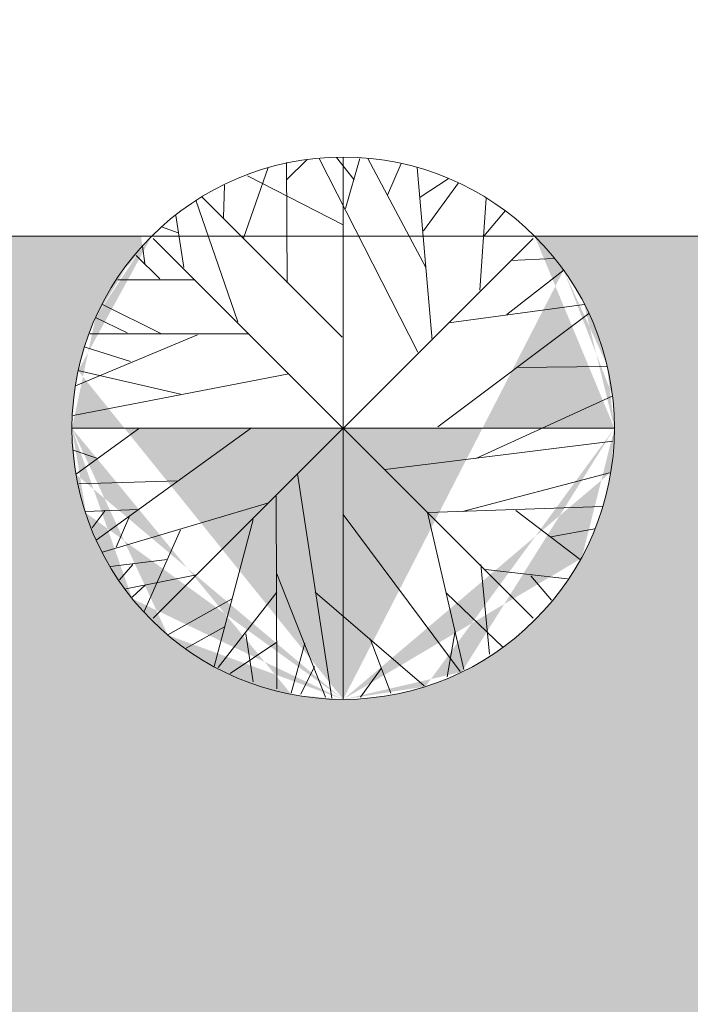
# Model space of a CAD drawing. Units: inches. Extents: x 459864 to 460310, y 324185 to 324787.
# Tile 62 of 112: x 460180 to 460210, y 324239 to 324282. Entities that reach past the tile are written whole.
import ezdxf

# ---------------------------------------------------------------- set-up
doc = ezdxf.new("R2010")
doc.units = ezdxf.units.IN
doc.layers.add('L-PLNT', color=3, linetype='Continuous', lineweight=13)
doc.layers.add('L-SITE-PATT', color=252, linetype='Continuous', lineweight=13)

# ---------------------------------------------------------------- blocks, each defined once
blk = doc.blocks.new('Tree - deciduous plan')
for p, q in [((-12.5388, 54.9406), (-7.9613, 59.4546)), ((-5.3205, 59.6806), (16.5105, 16.7963)), ((2.426, 54.9406), (-1.4472, 59.9056)), ((0, 59.9996), (0, -60)), ((0.4894, 48.6208), (3.6584, 59.6806)), ((18.2711, 35.5298), (5.419, 59.6806)), ((-22.0458, 42.0753), (-16.5881, 57.6486)), ((-12.3627, 32.1443), (-12.5388, 58.7776)), ((9.8203, 51.5549), (12.8133, 58.5516)), ((19.6795, 19.5047), (16.3344, 57.6486)), ((-21.1656, 55.8436), (-0.0388, 45.0094)), ((17.0387, 51.1035), (23.2006, 55.1666)), ((-26.4472, 46.5894), (-26.2712, 53.8116)), ((17.7429, 43.6552), (25.4894, 54.2636)), ((-32.6092, 50.4264), (-23.2782, 23.5674)), ((-31.2008, 51.1035), (-0.2149, 20.1818)), ((31.6513, 50.8778), (30.2429, 30.5643)), ((31.1232, 42.5267), (35.8767, 48.1693)), ((-37.0107, 47.0408), (-35.25, 35.5298)), ((-40.1797, 44.558), (-36.4825, 43.2038)), ((42, 42), (-42, -42)), ((42, -42), (-42, 42)), ((-43.8768, 36.4326), (-44.405, 40.2696)), ((-45.8134, 38.2383), (-40.5318, 33.0471)), ((37.1091, 37.1098), (46.6161, 37.5612)), ((36.2288, 25.1474), (48.9049, 35.0784)), ((-49.8627, 32.8214), (-32.7853, 32.8214)), ((-53.2078, 27.4044), (-40.1797, 20.859)), ((23.3767, 23.3417), (53.3063, 27.4044)), ((-54.7923, 24.4702), (-47.75, 21.0847)), ((54.3626, 25.3731), (20.9119, 0.3198)), ((-32.2571, 20.6333), (-59.1937, 9.348)), ((-56.0247, 20.859), (-20.8134, 20.859)), ((-57.081, 17.9248), (-47.0458, 14.7649)), ((38.5175, 13.4107), (58.2359, 13.6364)), ((-59.7219, 2.8025), (-12.0106, 12.0565)), ((-58.6656, 12.7336), (-35.9543, 7.5424)), ((29.3626, -6.6771), (59.4682, 7.091)), ((-54.6162, -24.7335), (-20.2853, 0.0941)), ((-60, 0), (60, 0)), ((-45.2853, -0.1316), (-59.0177, -10.0627)), ((9.2922, -9.1598), (59.6443, -2.8401)), ((-59.7219, -4.8714), (-54.2641, -6.6771)), ((-10.074, -10.0627), (-2.5036, -59.7178)), ((26.3697, -18.4138), (58.9401, -9.8369)), ((-58.4895, -12.3197), (-36.4825, -11.6426)), ((-14.8275, -15.0282), (-14.6515, -57.6865)), ((-53.2078, -27.442), (-16.7641, -16.6081)), ((18.7992, -18.6394), (57.3556, -17.2853)), ((-57.081, -18.4138), (-45.2853, -17.9624)), ((-52.6797, -18.188), (-55.4966, -22.0251)), ((-47.2219, -19.3166), (-50.2148, -26.3135)), ((-0.0388, -19.0909), (25.8415, -53.8495)), ((18.6232, -18.6394), (26.7218, -53.3981)), ((38.1654, -18.188), (52.426, -29.0219)), ((-19.9331, -20.2194), (-28.5599, -52.721)), ((-35.9543, -22.4765), (-44.0529, -40.5329)), ((45.9119, -24.0564), (55.595, -22.2508)), ((-38.9472, -29.0219), (-51.4472, -30.6018)), ((-46.5177, -30.1504), (-49.5106, -33.536)), ((30.419, -30.1504), (32.3556, -50.0125)), ((-32.4331, -32.4075), (-48.1021, -35.5674)), ((-14.6515, -32.1818), (-3.912, -59.4922)), ((31.4753, -31.279), (49.6091, -33.3103)), ((41.5105, -32.6332), (46.088, -38.0501)), ((-43.7008, -34.6645), (-46.6937, -37.373)), ((-14.6515, -36.2445), (-27.6797, -52.9467)), ((-6.2008, -36.2445), (17.919, -57.0094)), ((22.8485, -36.4702), (35.3485, -48.4326)), ((-24.6867, -37.8244), (-38.7712, -45.7241)), ((-26.2712, -43.9185), (-34.7219, -48.6583)), ((-21.5177, -45.4984), (-19.9331, -56.1065)), ((24.7852, -44.8213), (23.0246, -54.978)), ((-14.6515, -47.3041), (-25.0388, -54.3009)), ((-8.4895, -47.5298), (-11.4825, -58.5893)), ((5.9471, -46.6269), (10.5246, -58.5893)), ((-6.3768, -52.721), (-9.3698, -58.815)), ((8.4119, -53.1724), (3.8344, -59.4922))]:
    blk.add_line(p, q)
blk.add_circle((0, 0), 60)

msp = doc.modelspace()

# ---------------------------------------------------------------- hatches: boundary and pattern name
at = {"layer": 'L-SITE-PATT'}
h = msp.add_hatch(dxfattribs=at)
h.set_pattern_fill('DOTS', color=256)
h.paths.add_polyline_path([(460269.804, 324283.483), (460247.115, 324283.483), (460121.929, 324283.483), (460121.929, 324252.473), (460117.429, 324252.473), (460110.124, 324252.473), (460110.124, 324243.287), (460080.83, 324243.287), (460080.83, 324252.473), (460061.115, 324252.473), (460061.115, 324251.882), (460077.909, 324251.882), (460077.909, 324199.483), (460080.83, 324199.483), (460080.83, 324207.553), (460110.124, 324207.553), (460110.124, 324199.483), (460110.813, 324199.483), (460262.115, 324199.483), (460269.804, 324199.483)], flags=17)
edge = h.paths.add_edge_path(flags=0)
edge.add_ellipse((460222.59, 324263.813), major_axis=(-8.485, 8.485), ratio=1, start_angle=405, end_angle=495, ccw=False)
edge.add_line((460214.821, 324254.66), (460214.832, 324254.666))
edge.add_ellipse((460222.59, 324263.813), major_axis=(-8.485, 8.485), ratio=1, start_angle=405, end_angle=495, ccw=False)
edge.add_line((460210.759, 324261.781), (460210.768, 324261.787))
edge.add_ellipse((460222.59, 324263.813), major_axis=(-8.485, 8.485), ratio=1, start_angle=405, end_angle=495, ccw=False)
edge.add_ellipse((460222.59, 324263.813), major_axis=(-8.485, 8.485), ratio=1, start_angle=392.754, end_angle=405, ccw=False)
edge.add_ellipse((460222.59, 324263.813), major_axis=(-8.485, 8.485), ratio=1, start_angle=380.9347, end_angle=392.754, ccw=False)
edge.add_line((460211.337, 324267.985), (460211.34, 324267.985))
edge.add_ellipse((460222.59, 324263.813), major_axis=(-8.485, 8.485), ratio=1, start_angle=380.9347, end_angle=392.754, ccw=False)
edge.add_ellipse((460222.59, 324263.813), major_axis=(-8.485, 8.485), ratio=1, start_angle=347.9015, end_angle=380.9347, ccw=False)
edge.add_ellipse((460222.59, 324263.813), major_axis=(-8.485, 8.485), ratio=1, start_angle=327.0619, end_angle=347.9015, ccw=False)
edge.add_ellipse((460222.59, 324263.813), major_axis=(-8.485, 8.485), ratio=1, start_angle=278.3246, end_angle=327.0619, ccw=False)
edge.add_line((460225.158, 324275.536), (460225.158, 324275.535))
edge.add_ellipse((460222.59, 324263.813), major_axis=(-8.485, 8.485), ratio=1, start_angle=278.3246, end_angle=327.0619, ccw=False)
edge.add_ellipse((460222.59, 324263.813), major_axis=(-8.485, 8.485), ratio=1, start_angle=260.6436, end_angle=278.3246, ccw=False)
edge.add_ellipse((460222.59, 324263.813), major_axis=(-8.485, 8.485), ratio=1, start_angle=225, end_angle=260.6436, ccw=False)
edge.add_line((460234.509, 324265.243), (460234.501, 324265.239))
edge.add_ellipse((460222.59, 324263.813), major_axis=(-8.485, 8.485), ratio=1, start_angle=225, end_angle=260.6436, ccw=False)
edge.add_ellipse((460222.59, 324263.813), major_axis=(-8.485, 8.485), ratio=1, start_angle=495, end_angle=585, ccw=False)
edge.add_line((460234.437, 324261.861), (460234.424, 324261.858))
edge.add_ellipse((460222.59, 324263.813), major_axis=(-8.485, 8.485), ratio=1, start_angle=495, end_angle=585, ccw=False)
edge.add_line((460227.95, 324253.067), (460227.946, 324253.083))
edge.add_ellipse((460222.59, 324263.813), major_axis=(-8.485, 8.485), ratio=1, start_angle=495, end_angle=585, ccw=False)
edge.add_line((460226.223, 324252.369), (460226.211, 324252.38))
edge.add_ellipse((460222.59, 324263.813), major_axis=(-8.485, 8.485), ratio=1, start_angle=495, end_angle=585, ccw=False)
h.paths.add_polyline_path([(460219.651, 324254.347), (460218.461, 324253.545), (460218.275, 324254.789), (460219.642, 324256.542), (460219.625, 324260.848), (460216.11, 324257.333), (460214.35, 324256.978), (460215.416, 324259.356), (460212.524, 324258.496), (460213.137, 324259.93), (460218.507, 324263.813), (460222.59, 324263.813), (460222.59, 324267.807), (460218.176, 324272.212), (460219.026, 324274.639), (460222.59, 324272.811), (460222.59, 324275.423), (460223.057, 324274.825), (460222.675, 324273.492), (460225.912, 324267.135), (460219.625, 324260.848)], flags=0)
edge = h.paths.add_edge_path(flags=0)
edge.add_ellipse((460194.576, 324264.046), major_axis=(-8.485, 8.485), ratio=1, start_angle=495, end_angle=585, ccw=False)
edge.add_line((460199.936, 324253.3), (460199.932, 324253.316))
edge.add_ellipse((460194.576, 324264.046), major_axis=(-8.485, 8.485), ratio=1, start_angle=495, end_angle=585, ccw=False)
edge.add_line((460198.208, 324252.603), (460198.196, 324252.613))
edge.add_ellipse((460194.576, 324264.046), major_axis=(-8.485, 8.485), ratio=1, start_angle=495, end_angle=585, ccw=False)
edge.add_ellipse((460194.576, 324264.046), major_axis=(-8.485, 8.485), ratio=1, start_angle=405, end_angle=495, ccw=False)
edge.add_line((460186.806, 324254.893), (460186.817, 324254.899))
edge.add_ellipse((460194.576, 324264.046), major_axis=(-8.485, 8.485), ratio=1, start_angle=405, end_angle=495, ccw=False)
edge.add_line((460182.744, 324262.014), (460182.753, 324262.02))
edge.add_ellipse((460194.576, 324264.046), major_axis=(-8.485, 8.485), ratio=1, start_angle=405, end_angle=495, ccw=False)
edge.add_ellipse((460194.576, 324264.046), major_axis=(-8.485, 8.485), ratio=1, start_angle=392.754, end_angle=405, ccw=False)
edge.add_ellipse((460194.576, 324264.046), major_axis=(-8.485, 8.485), ratio=1, start_angle=380.9347, end_angle=392.754, ccw=False)
edge.add_line((460183.323, 324268.218), (460183.326, 324268.218))
edge.add_ellipse((460194.576, 324264.046), major_axis=(-8.485, 8.485), ratio=1, start_angle=380.9347, end_angle=392.754, ccw=False)
edge.add_ellipse((460194.576, 324264.046), major_axis=(-8.485, 8.485), ratio=1, start_angle=347.9015, end_angle=380.9347, ccw=False)
edge.add_ellipse((460194.576, 324264.046), major_axis=(-8.485, 8.485), ratio=1, start_angle=327.0619, end_angle=347.9015, ccw=False)
edge.add_ellipse((460194.576, 324264.046), major_axis=(-8.485, 8.485), ratio=1, start_angle=278.3246, end_angle=327.0619, ccw=False)
edge.add_line((460197.144, 324275.769), (460197.143, 324275.768))
edge.add_ellipse((460194.576, 324264.046), major_axis=(-8.485, 8.485), ratio=1, start_angle=278.3246, end_angle=327.0619, ccw=False)
edge.add_ellipse((460194.576, 324264.046), major_axis=(-8.485, 8.485), ratio=1, start_angle=260.6436, end_angle=278.3246, ccw=False)
edge.add_ellipse((460194.576, 324264.046), major_axis=(-8.485, 8.485), ratio=1, start_angle=225, end_angle=260.6436, ccw=False)
edge.add_line((460206.494, 324265.476), (460206.487, 324265.473))
edge.add_ellipse((460194.576, 324264.046), major_axis=(-8.485, 8.485), ratio=1, start_angle=225, end_angle=260.6436, ccw=False)
edge.add_ellipse((460194.576, 324264.046), major_axis=(-8.485, 8.485), ratio=1, start_angle=495, end_angle=585, ccw=False)
edge.add_line((460206.422, 324262.094), (460206.409, 324262.091))
h.paths.add_polyline_path([(460191.61, 324261.081), (460191.637, 324254.58), (460190.447, 324253.778), (460190.261, 324255.023), (460191.628, 324256.775), (460191.61, 324261.081), (460188.096, 324257.566), (460186.335, 324257.211), (460187.402, 324259.589), (460184.509, 324258.729), (460185.123, 324260.163), (460190.493, 324264.046), (460194.576, 324264.046), (460194.576, 324268.04), (460190.161, 324272.446), (460191.011, 324274.872), (460194.576, 324273.044), (460194.576, 324275.657), (460195.043, 324275.058), (460194.661, 324273.725), (460197.897, 324267.368)], flags=0)
edge = h.paths.add_edge_path(flags=0)
edge.add_ellipse((460252.912, 324263.578), major_axis=(-8.485, 8.485), ratio=1, start_angle=405, end_angle=495, ccw=False)
edge.add_line((460241.081, 324261.545), (460241.089, 324261.551))
edge.add_ellipse((460252.912, 324263.578), major_axis=(-8.485, 8.485), ratio=1, start_angle=405, end_angle=495, ccw=False)
edge.add_ellipse((460252.912, 324263.578), major_axis=(-8.485, 8.485), ratio=1, start_angle=392.754, end_angle=405, ccw=False)
edge.add_ellipse((460252.912, 324263.578), major_axis=(-8.485, 8.485), ratio=1, start_angle=380.9347, end_angle=392.754, ccw=False)
edge.add_line((460241.659, 324267.749), (460241.662, 324267.749))
edge.add_ellipse((460252.912, 324263.578), major_axis=(-8.485, 8.485), ratio=1, start_angle=380.9347, end_angle=392.754, ccw=False)
edge.add_ellipse((460252.912, 324263.578), major_axis=(-8.485, 8.485), ratio=1, start_angle=347.9015, end_angle=380.9347, ccw=False)
edge.add_ellipse((460252.912, 324263.578), major_axis=(-8.485, 8.485), ratio=1, start_angle=327.0619, end_angle=347.9015, ccw=False)
edge.add_ellipse((460252.912, 324263.578), major_axis=(-8.485, 8.485), ratio=1, start_angle=278.3246, end_angle=327.0619, ccw=False)
edge.add_line((460255.48, 324275.3), (460255.479, 324275.299))
edge.add_ellipse((460252.912, 324263.578), major_axis=(-8.485, 8.485), ratio=1, start_angle=278.3246, end_angle=327.0619, ccw=False)
edge.add_ellipse((460252.912, 324263.578), major_axis=(-8.485, 8.485), ratio=1, start_angle=260.6436, end_angle=278.3246, ccw=False)
edge.add_ellipse((460252.912, 324263.578), major_axis=(-8.485, 8.485), ratio=1, start_angle=225, end_angle=260.6436, ccw=False)
edge.add_line((460264.83, 324265.007), (460264.823, 324265.004))
edge.add_ellipse((460252.912, 324263.578), major_axis=(-8.485, 8.485), ratio=1, start_angle=225, end_angle=260.6436, ccw=False)
edge.add_ellipse((460252.912, 324263.578), major_axis=(-8.485, 8.485), ratio=1, start_angle=495, end_angle=585, ccw=False)
edge.add_line((460264.758, 324261.626), (460264.745, 324261.622))
edge.add_ellipse((460252.912, 324263.578), major_axis=(-8.485, 8.485), ratio=1, start_angle=495, end_angle=585, ccw=False)
edge.add_line((460258.272, 324252.832), (460258.268, 324252.848))
edge.add_ellipse((460252.912, 324263.578), major_axis=(-8.485, 8.485), ratio=1, start_angle=495, end_angle=585, ccw=False)
edge.add_line((460256.545, 324252.134), (460256.533, 324252.144))
edge.add_ellipse((460252.912, 324263.578), major_axis=(-8.485, 8.485), ratio=1, start_angle=495, end_angle=585, ccw=False)
edge.add_ellipse((460252.912, 324263.578), major_axis=(-8.485, 8.485), ratio=1, start_angle=405, end_angle=495, ccw=False)
edge.add_line((460245.143, 324254.424), (460245.153, 324254.43))
h.paths.add_polyline_path([(460244.672, 324256.742), (460245.738, 324259.12), (460242.846, 324258.26), (460243.459, 324259.694), (460248.829, 324263.578), (460252.912, 324263.578), (460252.912, 324267.571), (460248.497, 324271.977), (460249.348, 324274.403), (460252.912, 324272.576), (460252.912, 324275.188), (460253.379, 324274.589), (460252.997, 324273.257), (460256.233, 324266.899), (460249.946, 324260.612), (460249.973, 324254.111), (460248.783, 324253.309), (460248.597, 324254.554), (460249.964, 324256.306), (460249.946, 324260.612), (460246.432, 324257.097)], flags=0)
edge = h.paths.add_edge_path(flags=0)
edge.add_ellipse((460167.439, 324262.833), major_axis=(-8.485, 8.485), ratio=1, start_angle=495, end_angle=585, ccw=False)
edge.add_line((460172.799, 324252.087), (460172.795, 324252.103))
edge.add_ellipse((460167.439, 324262.833), major_axis=(-8.485, 8.485), ratio=1, start_angle=495, end_angle=585, ccw=False)
edge.add_line((460171.071, 324251.389), (460171.059, 324251.399))
edge.add_ellipse((460167.439, 324262.833), major_axis=(-8.485, 8.485), ratio=1, start_angle=495, end_angle=585, ccw=False)
edge.add_ellipse((460167.439, 324262.833), major_axis=(-8.485, 8.485), ratio=1, start_angle=405, end_angle=495, ccw=False)
edge.add_line((460159.669, 324253.679), (460159.68, 324253.685))
edge.add_ellipse((460167.439, 324262.833), major_axis=(-8.485, 8.485), ratio=1, start_angle=405, end_angle=495, ccw=False)
edge.add_line((460155.607, 324260.8), (460155.616, 324260.806))
edge.add_ellipse((460167.439, 324262.833), major_axis=(-8.485, 8.485), ratio=1, start_angle=405, end_angle=495, ccw=False)
edge.add_ellipse((460167.439, 324262.833), major_axis=(-8.485, 8.485), ratio=1, start_angle=392.754, end_angle=405, ccw=False)
edge.add_ellipse((460167.439, 324262.833), major_axis=(-8.485, 8.485), ratio=1, start_angle=380.9347, end_angle=392.754, ccw=False)
edge.add_line((460156.185, 324267.005), (460156.189, 324267.005))
edge.add_ellipse((460167.439, 324262.833), major_axis=(-8.485, 8.485), ratio=1, start_angle=380.9347, end_angle=392.754, ccw=False)
edge.add_ellipse((460167.439, 324262.833), major_axis=(-8.485, 8.485), ratio=1, start_angle=347.9015, end_angle=380.9347, ccw=False)
edge.add_ellipse((460167.439, 324262.833), major_axis=(-8.485, 8.485), ratio=1, start_angle=327.0619, end_angle=347.9015, ccw=False)
edge.add_ellipse((460167.439, 324262.833), major_axis=(-8.485, 8.485), ratio=1, start_angle=278.3246, end_angle=327.0619, ccw=False)
edge.add_line((460170.007, 324274.556), (460170.006, 324274.554))
edge.add_ellipse((460167.439, 324262.833), major_axis=(-8.485, 8.485), ratio=1, start_angle=278.3246, end_angle=327.0619, ccw=False)
edge.add_ellipse((460167.439, 324262.833), major_axis=(-8.485, 8.485), ratio=1, start_angle=260.6436, end_angle=278.3246, ccw=False)
edge.add_ellipse((460167.439, 324262.833), major_axis=(-8.485, 8.485), ratio=1, start_angle=225, end_angle=260.6436, ccw=False)
edge.add_line((460179.357, 324264.262), (460179.35, 324264.259))
edge.add_ellipse((460167.439, 324262.833), major_axis=(-8.485, 8.485), ratio=1, start_angle=225, end_angle=260.6436, ccw=False)
edge.add_ellipse((460167.439, 324262.833), major_axis=(-8.485, 8.485), ratio=1, start_angle=495, end_angle=585, ccw=False)
edge.add_line((460179.285, 324260.881), (460179.272, 324260.877))
h.paths.add_polyline_path([(460164.473, 324259.867), (460164.5, 324253.366), (460163.31, 324252.565), (460163.124, 324253.809), (460164.491, 324255.561), (460164.473, 324259.867), (460160.958, 324256.353), (460159.198, 324255.998), (460160.265, 324258.375), (460157.372, 324257.515), (460157.986, 324258.949), (460163.356, 324262.833), (460167.439, 324262.833), (460167.439, 324266.826), (460163.024, 324271.232), (460163.874, 324273.659), (460167.439, 324271.831), (460167.439, 324274.443), (460167.905, 324273.844), (460167.524, 324272.512), (460170.76, 324266.154)], flags=0)
edge = h.paths.add_edge_path(flags=0)
edge.add_ellipse((460140.758, 324262.37), major_axis=(-8.485, 8.485), ratio=1, start_angle=495, end_angle=585, ccw=False)
edge.add_line((460146.118, 324251.624), (460146.114, 324251.639))
edge.add_ellipse((460140.758, 324262.37), major_axis=(-8.485, 8.485), ratio=1, start_angle=495, end_angle=585, ccw=False)
edge.add_line((460144.391, 324250.926), (460144.379, 324250.936))
edge.add_ellipse((460140.758, 324262.37), major_axis=(-8.485, 8.485), ratio=1, start_angle=495, end_angle=585, ccw=False)
edge.add_ellipse((460140.758, 324262.37), major_axis=(-8.485, 8.485), ratio=1, start_angle=405, end_angle=495, ccw=False)
edge.add_line((460132.989, 324253.216), (460132.999, 324253.222))
edge.add_ellipse((460140.758, 324262.37), major_axis=(-8.485, 8.485), ratio=1, start_angle=405, end_angle=495, ccw=False)
edge.add_line((460128.927, 324260.337), (460128.935, 324260.343))
edge.add_ellipse((460140.758, 324262.37), major_axis=(-8.485, 8.485), ratio=1, start_angle=405, end_angle=495, ccw=False)
edge.add_ellipse((460140.758, 324262.37), major_axis=(-8.485, 8.485), ratio=1, start_angle=392.754, end_angle=405, ccw=False)
edge.add_ellipse((460140.758, 324262.37), major_axis=(-8.485, 8.485), ratio=1, start_angle=380.9347, end_angle=392.754, ccw=False)
edge.add_line((460129.505, 324266.541), (460129.508, 324266.541))
edge.add_ellipse((460140.758, 324262.37), major_axis=(-8.485, 8.485), ratio=1, start_angle=380.9347, end_angle=392.754, ccw=False)
edge.add_ellipse((460140.758, 324262.37), major_axis=(-8.485, 8.485), ratio=1, start_angle=347.9015, end_angle=380.9347, ccw=False)
edge.add_ellipse((460140.758, 324262.37), major_axis=(-8.485, 8.485), ratio=1, start_angle=327.0619, end_angle=347.9015, ccw=False)
edge.add_ellipse((460140.758, 324262.37), major_axis=(-8.485, 8.485), ratio=1, start_angle=278.3246, end_angle=327.0619, ccw=False)
edge.add_line((460143.326, 324274.092), (460143.325, 324274.091))
edge.add_ellipse((460140.758, 324262.37), major_axis=(-8.485, 8.485), ratio=1, start_angle=278.3246, end_angle=327.0619, ccw=False)
edge.add_ellipse((460140.758, 324262.37), major_axis=(-8.485, 8.485), ratio=1, start_angle=260.6436, end_angle=278.3246, ccw=False)
edge.add_ellipse((460140.758, 324262.37), major_axis=(-8.485, 8.485), ratio=1, start_angle=225, end_angle=260.6436, ccw=False)
edge.add_line((460152.677, 324263.799), (460152.669, 324263.796))
edge.add_ellipse((460140.758, 324262.37), major_axis=(-8.485, 8.485), ratio=1, start_angle=225, end_angle=260.6436, ccw=False)
edge.add_ellipse((460140.758, 324262.37), major_axis=(-8.485, 8.485), ratio=1, start_angle=495, end_angle=585, ccw=False)
edge.add_line((460152.604, 324260.418), (460152.592, 324260.414))
h.paths.add_polyline_path([(460137.792, 324259.404), (460137.819, 324252.903), (460136.629, 324252.101), (460136.443, 324253.346), (460137.81, 324255.098), (460137.792, 324259.404), (460134.278, 324255.889), (460132.518, 324255.534), (460133.584, 324257.912), (460130.692, 324257.052), (460131.305, 324258.486), (460136.675, 324262.37), (460140.758, 324262.37), (460140.758, 324266.363), (460136.343, 324270.769), (460137.194, 324273.195), (460140.758, 324271.367), (460140.758, 324273.98), (460141.225, 324273.381), (460140.843, 324272.049), (460144.079, 324265.691)], flags=0)
h.paths.add_polyline_path([(460110.124, 324227.414), (460080.83, 324227.414), (460080.83, 324235.484), (460110.124, 324235.484)], flags=16)
h.paths.add_polyline_path([(460110.124, 324220.797), (460110.124, 324212.727), (460080.83, 324212.727), (460080.83, 324220.797)], flags=16)
h.paths.add_polyline_path([(460269.804, 324283.483), (460247.115, 324283.483), (460121.929, 324283.483), (460121.929, 324252.473), (460117.429, 324252.473), (460110.124, 324252.473), (460110.124, 324243.287), (460080.83, 324243.287), (460080.83, 324252.473), (460061.115, 324252.473), (460061.115, 324251.882), (460077.909, 324251.882), (460077.909, 324199.483), (460080.83, 324199.483), (460080.83, 324207.553), (460110.124, 324207.553), (460110.124, 324199.483), (460262.115, 324199.483), (460269.804, 324199.483)], flags=17)
h.paths.add_polyline_path([(460219.651, 324254.347), (460218.461, 324253.545), (460218.275, 324254.789), (460219.642, 324256.542), (460219.625, 324260.848), (460216.11, 324257.333), (460214.35, 324256.978), (460215.416, 324259.356), (460212.524, 324258.496), (460213.137, 324259.93), (460218.507, 324263.813), (460222.59, 324263.813), (460220.18, 324266.223), (460215.461, 324265.308), (460211.835, 324266.137), (460216.247, 324267.985), (460218.418, 324267.985), (460222.59, 324263.813), (460222.59, 324267.807), (460218.176, 324272.212), (460219.026, 324274.639), (460222.59, 324272.811), (460222.59, 324275.423), (460223.057, 324274.825), (460222.675, 324273.492), (460225.912, 324267.135), (460222.59, 324263.813), (460231.383, 324263.813), (460228.485, 324262.488), (460224.425, 324261.978), (460228.68, 324257.724), (460228.966, 324254.791), (460227.142, 324256.537), (460227.542, 324254.819), (460227.333, 324253.614), (460222.59, 324259.985), (460222.59, 324255.497), (460221.377, 324256.541), (460220.576, 324261.799), (460219.625, 324260.848)], flags=0)
h.paths.add_polyline_path([(460199.127, 324256.77), (460199.528, 324255.052), (460199.319, 324253.848), (460194.576, 324260.218), (460194.576, 324255.73), (460193.363, 324256.774), (460192.561, 324262.032), (460191.61, 324261.081), (460191.637, 324254.58), (460190.447, 324253.778), (460190.261, 324255.023), (460191.628, 324256.775), (460191.61, 324261.081), (460188.096, 324257.566), (460186.335, 324257.211), (460187.402, 324259.589), (460184.509, 324258.729), (460185.123, 324260.163), (460190.493, 324264.046), (460194.576, 324264.046), (460192.166, 324266.456), (460187.446, 324265.541), (460183.82, 324266.37), (460188.232, 324268.218), (460190.404, 324268.218), (460194.576, 324264.046), (460194.576, 324268.04), (460190.161, 324272.446), (460191.011, 324274.872), (460194.576, 324273.044), (460194.576, 324275.657), (460195.043, 324275.058), (460194.661, 324273.725), (460197.897, 324267.368), (460194.576, 324264.046), (460203.368, 324264.046), (460200.47, 324262.721), (460196.411, 324262.212), (460200.665, 324257.957), (460200.951, 324255.024)], flags=0)
h.paths.add_polyline_path([(460244.672, 324256.742), (460245.738, 324259.12), (460242.846, 324258.26), (460243.459, 324259.694), (460248.829, 324263.578), (460252.912, 324263.578), (460250.502, 324265.987), (460245.783, 324265.072), (460242.156, 324265.901), (460246.568, 324267.749), (460248.74, 324267.749), (460252.912, 324263.578), (460252.912, 324267.571), (460248.497, 324271.977), (460249.348, 324274.403), (460252.912, 324272.576), (460252.912, 324275.188), (460253.379, 324274.589), (460252.997, 324273.257), (460256.233, 324266.899), (460252.912, 324263.578), (460261.705, 324263.578), (460258.806, 324262.252), (460254.747, 324261.743), (460259.002, 324257.488), (460259.288, 324254.555), (460257.463, 324256.301), (460257.864, 324254.583), (460257.655, 324253.379), (460252.912, 324259.749), (460252.912, 324255.261), (460251.699, 324256.305), (460250.897, 324261.563), (460249.946, 324260.612), (460249.973, 324254.111), (460248.783, 324253.309), (460248.597, 324254.554), (460249.964, 324256.306), (460249.946, 324260.612), (460246.432, 324257.097)], flags=0)
h.paths.add_polyline_path([(460173.528, 324256.743), (460173.814, 324253.811), (460171.99, 324255.556), (460172.39, 324253.838), (460172.182, 324252.634), (460167.439, 324259.004), (460167.439, 324254.516), (460166.226, 324255.56), (460165.424, 324260.818), (460164.473, 324259.867), (460164.5, 324253.366), (460163.31, 324252.565), (460163.124, 324253.809), (460164.491, 324255.561), (460164.473, 324259.867), (460160.958, 324256.353), (460159.198, 324255.998), (460160.265, 324258.375), (460157.372, 324257.515), (460157.986, 324258.949), (460163.356, 324262.833), (460167.439, 324262.833), (460165.029, 324265.243), (460160.309, 324264.327), (460156.683, 324265.156), (460161.095, 324267.005), (460163.267, 324267.005), (460167.439, 324262.833), (460167.439, 324266.826), (460163.024, 324271.232), (460163.874, 324273.659), (460167.439, 324271.831), (460167.439, 324274.443), (460167.905, 324273.844), (460167.524, 324272.512), (460170.76, 324266.154), (460167.439, 324262.833), (460176.231, 324262.833), (460173.333, 324261.507), (460169.274, 324260.998)], flags=0)
h.paths.add_polyline_path([(460146.848, 324256.28), (460147.134, 324253.347), (460145.31, 324255.093), (460145.71, 324253.375), (460145.501, 324252.171), (460140.758, 324258.541), (460140.758, 324254.053), (460139.545, 324255.097), (460138.744, 324260.355), (460137.792, 324259.404), (460137.819, 324252.903), (460136.629, 324252.101), (460136.443, 324253.346), (460137.81, 324255.098), (460137.792, 324259.404), (460134.278, 324255.889), (460132.518, 324255.534), (460133.584, 324257.912), (460130.692, 324257.052), (460131.305, 324258.486), (460136.675, 324262.37), (460140.758, 324262.37), (460138.348, 324264.779), (460133.629, 324263.864), (460130.002, 324264.693), (460134.414, 324266.541), (460136.586, 324266.541), (460140.758, 324262.37), (460140.758, 324266.363), (460136.343, 324270.769), (460137.194, 324273.195), (460140.758, 324271.367), (460140.758, 324273.98), (460141.225, 324273.381), (460140.843, 324272.049), (460144.079, 324265.691), (460140.758, 324262.37), (460149.551, 324262.37), (460146.653, 324261.044), (460142.593, 324260.535)], flags=0)
edge = h.paths.add_edge_path()
edge.add_line((460269.804, 324272.549), (460260.881, 324272.549))
edge.add_ellipse((460252.912, 324263.578), major_axis=(-8.485, 8.485), ratio=1, start_angle=260.6436, end_angle=273.3846, ccw=False)
edge.add_line((460262.283, 324271.092), (460262.261, 324271.091))
edge.add_ellipse((460252.912, 324263.578), major_axis=(-8.485, 8.485), ratio=1, start_angle=260.6436, end_angle=273.3846, ccw=False)
edge.add_ellipse((460252.912, 324263.578), major_axis=(-8.485, 8.485), ratio=1, start_angle=225, end_angle=260.6436, ccw=False)
edge.add_line((460263.609, 324269.063), (460263.572, 324269.058))
edge.add_ellipse((460252.912, 324263.578), major_axis=(-8.485, 8.485), ratio=1, start_angle=225, end_angle=260.6436, ccw=False)
edge.add_line((460264.615, 324266.306), (460264.585, 324266.305))
edge.add_ellipse((460252.912, 324263.578), major_axis=(-8.485, 8.485), ratio=1, start_angle=225, end_angle=260.6436, ccw=False)
edge.add_line((460264.83, 324265.007), (460264.823, 324265.004))
edge.add_ellipse((460252.912, 324263.578), major_axis=(-8.485, 8.485), ratio=1, start_angle=225, end_angle=260.6436, ccw=False)
edge.add_ellipse((460252.912, 324263.578), major_axis=(-8.485, 8.485), ratio=1, start_angle=495, end_angle=585, ccw=False)
edge.add_line((460264.758, 324261.626), (460264.745, 324261.622))
edge.add_ellipse((460252.912, 324263.578), major_axis=(-8.485, 8.485), ratio=1, start_angle=495, end_angle=585, ccw=False)
edge.add_line((460263.442, 324257.739), (460263.389, 324257.779))
edge.add_ellipse((460252.912, 324263.578), major_axis=(-8.485, 8.485), ratio=1, start_angle=495, end_angle=585, ccw=False)
edge.add_line((460258.128, 324252.744), (460258.102, 324252.779))
edge.add_ellipse((460252.912, 324263.578), major_axis=(-8.485, 8.485), ratio=1, start_angle=495, end_angle=585, ccw=False)
edge.add_line((460256.545, 324252.134), (460256.533, 324252.144))
edge.add_ellipse((460252.912, 324263.578), major_axis=(-8.485, 8.485), ratio=1, start_angle=495, end_angle=585, ccw=False)
edge.add_ellipse((460252.912, 324263.578), major_axis=(-8.485, 8.485), ratio=1, start_angle=405, end_angle=495, ccw=False)
edge.add_line((460250.594, 324251.78), (460250.605, 324251.82))
edge.add_ellipse((460252.912, 324263.578), major_axis=(-8.485, 8.485), ratio=1, start_angle=405, end_angle=495, ccw=False)
edge.add_line((460245.143, 324254.424), (460245.153, 324254.43))
edge.add_ellipse((460252.912, 324263.578), major_axis=(-8.485, 8.485), ratio=1, start_angle=405, end_angle=495, ccw=False)
edge.add_line((460243.525, 324256.059), (460243.56, 324256.091))
edge.add_ellipse((460252.912, 324263.578), major_axis=(-8.485, 8.485), ratio=1, start_angle=405, end_angle=495, ccw=False)
edge.add_line((460241.44, 324259.893), (460241.522, 324259.896))
edge.add_ellipse((460252.912, 324263.578), major_axis=(-8.485, 8.485), ratio=1, start_angle=405, end_angle=495, ccw=False)
edge.add_line((460241.081, 324261.545), (460241.089, 324261.551))
edge.add_ellipse((460252.912, 324263.578), major_axis=(-8.485, 8.485), ratio=1, start_angle=405, end_angle=495, ccw=False)
edge.add_ellipse((460252.912, 324263.578), major_axis=(-8.485, 8.485), ratio=1, start_angle=392.754, end_angle=405, ccw=False)
edge.add_line((460241.05, 324265.438), (460241.063, 324265.443))
edge.add_ellipse((460252.912, 324263.578), major_axis=(-8.485, 8.485), ratio=1, start_angle=392.754, end_angle=405, ccw=False)
edge.add_ellipse((460252.912, 324263.578), major_axis=(-8.485, 8.485), ratio=1, start_angle=380.9347, end_angle=392.754, ccw=False)
edge.add_line((460241.452, 324267.176), (460241.469, 324267.171))
edge.add_ellipse((460252.912, 324263.578), major_axis=(-8.485, 8.485), ratio=1, start_angle=380.9347, end_angle=392.754, ccw=False)
edge.add_line((460241.659, 324267.749), (460241.662, 324267.749))
edge.add_ellipse((460252.912, 324263.578), major_axis=(-8.485, 8.485), ratio=1, start_angle=380.9347, end_angle=392.754, ccw=False)
edge.add_ellipse((460252.912, 324263.578), major_axis=(-8.485, 8.485), ratio=1, start_angle=356.6154, end_angle=380.9347, ccw=False)
edge.add_line((460244.88, 324272.488), (460244.713, 324272.549))
edge.add_line((460244.713, 324272.549), (460230.817, 324272.549))
edge.add_ellipse((460222.59, 324263.813), major_axis=(-8.485, 8.485), ratio=1, start_angle=260.6436, end_angle=271.7178, ccw=False)
edge.add_ellipse((460222.59, 324263.813), major_axis=(-8.485, 8.485), ratio=1, start_angle=225, end_angle=260.6436, ccw=False)
edge.add_line((460233.287, 324269.299), (460233.25, 324269.294))
edge.add_ellipse((460222.59, 324263.813), major_axis=(-8.485, 8.485), ratio=1, start_angle=225, end_angle=260.6436, ccw=False)
edge.add_line((460234.294, 324266.541), (460234.264, 324266.541))
edge.add_ellipse((460222.59, 324263.813), major_axis=(-8.485, 8.485), ratio=1, start_angle=225, end_angle=260.6436, ccw=False)
edge.add_line((460234.509, 324265.243), (460234.501, 324265.239))
edge.add_ellipse((460222.59, 324263.813), major_axis=(-8.485, 8.485), ratio=1, start_angle=225, end_angle=260.6436, ccw=False)
edge.add_ellipse((460222.59, 324263.813), major_axis=(-8.485, 8.485), ratio=1, start_angle=495, end_angle=585, ccw=False)
edge.add_line((460234.437, 324261.861), (460234.424, 324261.858))
edge.add_ellipse((460222.59, 324263.813), major_axis=(-8.485, 8.485), ratio=1, start_angle=495, end_angle=585, ccw=False)
edge.add_line((460233.121, 324257.975), (460233.068, 324258.015))
edge.add_ellipse((460222.59, 324263.813), major_axis=(-8.485, 8.485), ratio=1, start_angle=495, end_angle=585, ccw=False)
edge.add_line((460227.806, 324252.979), (460227.78, 324253.014))
edge.add_ellipse((460222.59, 324263.813), major_axis=(-8.485, 8.485), ratio=1, start_angle=495, end_angle=585, ccw=False)
edge.add_line((460226.223, 324252.369), (460226.211, 324252.38))
edge.add_ellipse((460222.59, 324263.813), major_axis=(-8.485, 8.485), ratio=1, start_angle=495, end_angle=585, ccw=False)
edge.add_ellipse((460222.59, 324263.813), major_axis=(-8.485, 8.485), ratio=1, start_angle=405, end_angle=495, ccw=False)
edge.add_line((460220.272, 324252.016), (460220.283, 324252.055))
edge.add_ellipse((460222.59, 324263.813), major_axis=(-8.485, 8.485), ratio=1, start_angle=405, end_angle=495, ccw=False)
edge.add_line((460214.821, 324254.66), (460214.832, 324254.666))
edge.add_ellipse((460222.59, 324263.813), major_axis=(-8.485, 8.485), ratio=1, start_angle=405, end_angle=495, ccw=False)
edge.add_line((460213.203, 324256.295), (460213.239, 324256.327))
edge.add_ellipse((460222.59, 324263.813), major_axis=(-8.485, 8.485), ratio=1, start_angle=405, end_angle=495, ccw=False)
edge.add_line((460211.118, 324260.128), (460211.201, 324260.131))
edge.add_ellipse((460222.59, 324263.813), major_axis=(-8.485, 8.485), ratio=1, start_angle=405, end_angle=495, ccw=False)
edge.add_line((460210.759, 324261.781), (460210.768, 324261.787))
edge.add_ellipse((460222.59, 324263.813), major_axis=(-8.485, 8.485), ratio=1, start_angle=405, end_angle=495, ccw=False)
edge.add_ellipse((460222.59, 324263.813), major_axis=(-8.485, 8.485), ratio=1, start_angle=392.754, end_angle=405, ccw=False)
edge.add_line((460210.729, 324265.673), (460210.741, 324265.678))
edge.add_ellipse((460222.59, 324263.813), major_axis=(-8.485, 8.485), ratio=1, start_angle=392.754, end_angle=405, ccw=False)
edge.add_ellipse((460222.59, 324263.813), major_axis=(-8.485, 8.485), ratio=1, start_angle=380.9347, end_angle=392.754, ccw=False)
edge.add_line((460211.13, 324267.412), (460211.147, 324267.407))
edge.add_ellipse((460222.59, 324263.813), major_axis=(-8.485, 8.485), ratio=1, start_angle=380.9347, end_angle=392.754, ccw=False)
edge.add_line((460211.337, 324267.985), (460211.34, 324267.985))
edge.add_ellipse((460222.59, 324263.813), major_axis=(-8.485, 8.485), ratio=1, start_angle=380.9347, end_angle=392.754, ccw=False)
edge.add_ellipse((460222.59, 324263.813), major_axis=(-8.485, 8.485), ratio=1, start_angle=358.2822, end_angle=380.9347, ccw=False)
edge.add_line((460213.705, 324271.902), (460213.709, 324271.869))
edge.add_ellipse((460222.59, 324263.813), major_axis=(-8.485, 8.485), ratio=1, start_angle=358.2822, end_angle=380.9347, ccw=False)
edge.add_line((460214.363, 324272.549), (460203.078, 324272.549))
edge.add_line((460203.078, 324272.549), (460203.06, 324272.531))
edge.add_ellipse((460194.576, 324264.046), major_axis=(-8.485, 8.485), ratio=1, start_angle=260.6436, end_angle=270.1168, ccw=False)
edge.add_line((460203.957, 324271.561), (460203.921, 324271.56))
edge.add_ellipse((460194.576, 324264.046), major_axis=(-8.485, 8.485), ratio=1, start_angle=260.6436, end_angle=270.1168, ccw=False)
edge.add_ellipse((460194.576, 324264.046), major_axis=(-8.485, 8.485), ratio=1, start_angle=225, end_angle=260.6436, ccw=False)
edge.add_line((460205.272, 324269.532), (460205.235, 324269.527))
edge.add_ellipse((460194.576, 324264.046), major_axis=(-8.485, 8.485), ratio=1, start_angle=225, end_angle=260.6436, ccw=False)
edge.add_line((460206.279, 324266.774), (460206.249, 324266.774))
edge.add_ellipse((460194.576, 324264.046), major_axis=(-8.485, 8.485), ratio=1, start_angle=225, end_angle=260.6436, ccw=False)
edge.add_line((460206.494, 324265.476), (460206.487, 324265.473))
edge.add_ellipse((460194.576, 324264.046), major_axis=(-8.485, 8.485), ratio=1, start_angle=225, end_angle=260.6436, ccw=False)
edge.add_ellipse((460194.576, 324264.046), major_axis=(-8.485, 8.485), ratio=1, start_angle=495, end_angle=585, ccw=False)
edge.add_line((460206.422, 324262.094), (460206.409, 324262.091))
edge.add_ellipse((460194.576, 324264.046), major_axis=(-8.485, 8.485), ratio=1, start_angle=495, end_angle=585, ccw=False)
edge.add_line((460205.106, 324258.208), (460205.053, 324258.248))
edge.add_ellipse((460194.576, 324264.046), major_axis=(-8.485, 8.485), ratio=1, start_angle=495, end_angle=585, ccw=False)
edge.add_line((460199.792, 324253.212), (460199.766, 324253.248))
edge.add_ellipse((460194.576, 324264.046), major_axis=(-8.485, 8.485), ratio=1, start_angle=495, end_angle=585, ccw=False)
edge.add_line((460198.208, 324252.603), (460198.196, 324252.613))
edge.add_ellipse((460194.576, 324264.046), major_axis=(-8.485, 8.485), ratio=1, start_angle=495, end_angle=585, ccw=False)
edge.add_ellipse((460194.576, 324264.046), major_axis=(-8.485, 8.485), ratio=1, start_angle=405, end_angle=495, ccw=False)
edge.add_line((460192.258, 324252.249), (460192.268, 324252.289))
edge.add_ellipse((460194.576, 324264.046), major_axis=(-8.485, 8.485), ratio=1, start_angle=405, end_angle=495, ccw=False)
edge.add_line((460186.806, 324254.893), (460186.817, 324254.899))
edge.add_ellipse((460194.576, 324264.046), major_axis=(-8.485, 8.485), ratio=1, start_angle=405, end_angle=495, ccw=False)
edge.add_line((460185.188, 324256.528), (460185.224, 324256.56))
edge.add_ellipse((460194.576, 324264.046), major_axis=(-8.485, 8.485), ratio=1, start_angle=405, end_angle=495, ccw=False)
edge.add_line((460183.104, 324260.362), (460183.186, 324260.365))
edge.add_ellipse((460194.576, 324264.046), major_axis=(-8.485, 8.485), ratio=1, start_angle=405, end_angle=495, ccw=False)
edge.add_line((460182.744, 324262.014), (460182.753, 324262.02))
edge.add_ellipse((460194.576, 324264.046), major_axis=(-8.485, 8.485), ratio=1, start_angle=405, end_angle=495, ccw=False)
edge.add_ellipse((460194.576, 324264.046), major_axis=(-8.485, 8.485), ratio=1, start_angle=392.754, end_angle=405, ccw=False)
edge.add_line((460182.714, 324265.906), (460182.726, 324265.912))
edge.add_ellipse((460194.576, 324264.046), major_axis=(-8.485, 8.485), ratio=1, start_angle=392.754, end_angle=405, ccw=False)
edge.add_ellipse((460194.576, 324264.046), major_axis=(-8.485, 8.485), ratio=1, start_angle=380.9347, end_angle=392.754, ccw=False)
edge.add_line((460183.116, 324267.645), (460183.133, 324267.64))
edge.add_ellipse((460194.576, 324264.046), major_axis=(-8.485, 8.485), ratio=1, start_angle=380.9347, end_angle=392.754, ccw=False)
edge.add_line((460183.323, 324268.218), (460183.326, 324268.218))
edge.add_ellipse((460194.576, 324264.046), major_axis=(-8.485, 8.485), ratio=1, start_angle=380.9347, end_angle=392.754, ccw=False)
edge.add_ellipse((460194.576, 324264.046), major_axis=(-8.485, 8.485), ratio=1, start_angle=359.8832, end_angle=380.9347, ccw=False)
edge.add_line((460184.491, 324270.611), (460184.553, 324270.611))
edge.add_ellipse((460194.576, 324264.046), major_axis=(-8.485, 8.485), ratio=1, start_angle=359.8832, end_angle=380.9347, ccw=False)
edge.add_line((460185.346, 324271.76), (460185.379, 324271.728))
edge.add_ellipse((460194.576, 324264.046), major_axis=(-8.485, 8.485), ratio=1, start_angle=359.8832, end_angle=380.9347, ccw=False)
edge.add_line((460185.697, 324272.086), (460185.633, 324272.549))
edge.add_line((460185.633, 324272.549), (460174.683, 324272.549))
edge.add_line((460174.683, 324272.549), (460174.606, 324272.457))
edge.add_ellipse((460167.439, 324262.833), major_axis=(-8.485, 8.485), ratio=1, start_angle=260.6436, end_angle=278.3246, ccw=False)
edge.add_ellipse((460167.439, 324262.833), major_axis=(-8.485, 8.485), ratio=1, start_angle=225, end_angle=260.6436, ccw=False)
edge.add_line((460178.135, 324268.318), (460178.098, 324268.313))
edge.add_ellipse((460167.439, 324262.833), major_axis=(-8.485, 8.485), ratio=1, start_angle=225, end_angle=260.6436, ccw=False)
edge.add_line((460179.142, 324265.561), (460179.112, 324265.56))
edge.add_ellipse((460167.439, 324262.833), major_axis=(-8.485, 8.485), ratio=1, start_angle=225, end_angle=260.6436, ccw=False)
edge.add_line((460179.357, 324264.262), (460179.35, 324264.259))
edge.add_ellipse((460167.439, 324262.833), major_axis=(-8.485, 8.485), ratio=1, start_angle=225, end_angle=260.6436, ccw=False)
edge.add_ellipse((460167.439, 324262.833), major_axis=(-8.485, 8.485), ratio=1, start_angle=495, end_angle=585, ccw=False)
edge.add_line((460179.285, 324260.881), (460179.272, 324260.877))
edge.add_ellipse((460167.439, 324262.833), major_axis=(-8.485, 8.485), ratio=1, start_angle=495, end_angle=585, ccw=False)
edge.add_line((460177.969, 324256.994), (460177.916, 324257.034))
edge.add_ellipse((460167.439, 324262.833), major_axis=(-8.485, 8.485), ratio=1, start_angle=495, end_angle=585, ccw=False)
edge.add_line((460172.655, 324251.999), (460172.629, 324252.034))
edge.add_ellipse((460167.439, 324262.833), major_axis=(-8.485, 8.485), ratio=1, start_angle=495, end_angle=585, ccw=False)
edge.add_line((460171.071, 324251.389), (460171.059, 324251.399))
edge.add_ellipse((460167.439, 324262.833), major_axis=(-8.485, 8.485), ratio=1, start_angle=495, end_angle=585, ccw=False)
edge.add_ellipse((460167.439, 324262.833), major_axis=(-8.485, 8.485), ratio=1, start_angle=405, end_angle=495, ccw=False)
edge.add_line((460165.121, 324251.036), (460165.131, 324251.075))
edge.add_ellipse((460167.439, 324262.833), major_axis=(-8.485, 8.485), ratio=1, start_angle=405, end_angle=495, ccw=False)
edge.add_line((460159.669, 324253.679), (460159.68, 324253.685))
edge.add_ellipse((460167.439, 324262.833), major_axis=(-8.485, 8.485), ratio=1, start_angle=405, end_angle=495, ccw=False)
edge.add_line((460158.051, 324255.314), (460158.087, 324255.347))
edge.add_ellipse((460167.439, 324262.833), major_axis=(-8.485, 8.485), ratio=1, start_angle=405, end_angle=495, ccw=False)
edge.add_line((460155.967, 324259.148), (460156.049, 324259.151))
edge.add_ellipse((460167.439, 324262.833), major_axis=(-8.485, 8.485), ratio=1, start_angle=405, end_angle=495, ccw=False)
edge.add_line((460155.607, 324260.8), (460155.616, 324260.806))
edge.add_ellipse((460167.439, 324262.833), major_axis=(-8.485, 8.485), ratio=1, start_angle=405, end_angle=495, ccw=False)
edge.add_ellipse((460167.439, 324262.833), major_axis=(-8.485, 8.485), ratio=1, start_angle=392.754, end_angle=405, ccw=False)
edge.add_line((460155.577, 324264.693), (460155.589, 324264.698))
edge.add_ellipse((460167.439, 324262.833), major_axis=(-8.485, 8.485), ratio=1, start_angle=392.754, end_angle=405, ccw=False)
edge.add_ellipse((460167.439, 324262.833), major_axis=(-8.485, 8.485), ratio=1, start_angle=380.9347, end_angle=392.754, ccw=False)
edge.add_line((460155.979, 324266.432), (460155.996, 324266.426))
edge.add_ellipse((460167.439, 324262.833), major_axis=(-8.485, 8.485), ratio=1, start_angle=380.9347, end_angle=392.754, ccw=False)
edge.add_line((460156.185, 324267.005), (460156.189, 324267.005))
edge.add_ellipse((460167.439, 324262.833), major_axis=(-8.485, 8.485), ratio=1, start_angle=380.9347, end_angle=392.754, ccw=False)
edge.add_ellipse((460167.439, 324262.833), major_axis=(-8.485, 8.485), ratio=1, start_angle=350.9345, end_angle=380.9347, ccw=False)
edge.add_line((460157.363, 324269.397), (460157.414, 324269.397))
edge.add_ellipse((460167.439, 324262.833), major_axis=(-8.485, 8.485), ratio=1, start_angle=350.9345, end_angle=380.9347, ccw=False)
edge.add_line((460158.221, 324270.535), (460158.236, 324270.519))
edge.add_ellipse((460167.439, 324262.833), major_axis=(-8.485, 8.485), ratio=1, start_angle=350.9345, end_angle=380.9347, ccw=False)
edge.add_line((460159.379, 324271.753), (460159.419, 324271.738))
edge.add_ellipse((460167.439, 324262.833), major_axis=(-8.485, 8.485), ratio=1, start_angle=350.9345, end_angle=380.9347, ccw=False)
edge.add_line((460160.396, 324272.549), (460147.112, 324272.549))
edge.add_ellipse((460140.758, 324262.37), major_axis=(-8.485, 8.485), ratio=1, start_angle=278.3246, end_angle=283.0261, ccw=False)
edge.add_ellipse((460140.758, 324262.37), major_axis=(-8.485, 8.485), ratio=1, start_angle=260.6436, end_angle=278.3246, ccw=False)
edge.add_ellipse((460140.758, 324262.37), major_axis=(-8.485, 8.485), ratio=1, start_angle=225, end_angle=260.6436, ccw=False)
edge.add_line((460151.455, 324267.855), (460151.418, 324267.85))
edge.add_ellipse((460140.758, 324262.37), major_axis=(-8.485, 8.485), ratio=1, start_angle=225, end_angle=260.6436, ccw=False)
edge.add_line((460152.462, 324265.098), (460152.431, 324265.097))
edge.add_ellipse((460140.758, 324262.37), major_axis=(-8.485, 8.485), ratio=1, start_angle=225, end_angle=260.6436, ccw=False)
edge.add_line((460152.677, 324263.799), (460152.669, 324263.796))
edge.add_ellipse((460140.758, 324262.37), major_axis=(-8.485, 8.485), ratio=1, start_angle=225, end_angle=260.6436, ccw=False)
edge.add_ellipse((460140.758, 324262.37), major_axis=(-8.485, 8.485), ratio=1, start_angle=495, end_angle=585, ccw=False)
edge.add_line((460152.604, 324260.418), (460152.592, 324260.414))
edge.add_ellipse((460140.758, 324262.37), major_axis=(-8.485, 8.485), ratio=1, start_angle=495, end_angle=585, ccw=False)
edge.add_line((460151.288, 324256.531), (460151.235, 324256.571))
edge.add_ellipse((460140.758, 324262.37), major_axis=(-8.485, 8.485), ratio=1, start_angle=495, end_angle=585, ccw=False)
edge.add_line((460145.974, 324251.535), (460145.948, 324251.571))
edge.add_ellipse((460140.758, 324262.37), major_axis=(-8.485, 8.485), ratio=1, start_angle=495, end_angle=585, ccw=False)
edge.add_line((460144.391, 324250.926), (460144.379, 324250.936))
edge.add_ellipse((460140.758, 324262.37), major_axis=(-8.485, 8.485), ratio=1, start_angle=495, end_angle=585, ccw=False)
edge.add_ellipse((460140.758, 324262.37), major_axis=(-8.485, 8.485), ratio=1, start_angle=405, end_angle=495, ccw=False)
edge.add_line((460138.44, 324250.572), (460138.451, 324250.612))
edge.add_ellipse((460140.758, 324262.37), major_axis=(-8.485, 8.485), ratio=1, start_angle=405, end_angle=495, ccw=False)
edge.add_line((460132.989, 324253.216), (460132.999, 324253.222))
edge.add_ellipse((460140.758, 324262.37), major_axis=(-8.485, 8.485), ratio=1, start_angle=405, end_angle=495, ccw=False)
edge.add_line((460131.371, 324254.851), (460131.406, 324254.883))
edge.add_ellipse((460140.758, 324262.37), major_axis=(-8.485, 8.485), ratio=1, start_angle=405, end_angle=495, ccw=False)
edge.add_line((460129.286, 324258.685), (460129.369, 324258.688))
edge.add_ellipse((460140.758, 324262.37), major_axis=(-8.485, 8.485), ratio=1, start_angle=405, end_angle=495, ccw=False)
edge.add_line((460128.927, 324260.337), (460128.935, 324260.343))
edge.add_ellipse((460140.758, 324262.37), major_axis=(-8.485, 8.485), ratio=1, start_angle=405, end_angle=495, ccw=False)
edge.add_ellipse((460140.758, 324262.37), major_axis=(-8.485, 8.485), ratio=1, start_angle=392.754, end_angle=405, ccw=False)
edge.add_line((460128.896, 324264.23), (460128.909, 324264.235))
edge.add_ellipse((460140.758, 324262.37), major_axis=(-8.485, 8.485), ratio=1, start_angle=392.754, end_angle=405, ccw=False)
edge.add_ellipse((460140.758, 324262.37), major_axis=(-8.485, 8.485), ratio=1, start_angle=380.9347, end_angle=392.754, ccw=False)
edge.add_line((460129.298, 324265.968), (460129.315, 324265.963))
edge.add_ellipse((460140.758, 324262.37), major_axis=(-8.485, 8.485), ratio=1, start_angle=380.9347, end_angle=392.754, ccw=False)
edge.add_line((460129.505, 324266.541), (460129.508, 324266.541))
edge.add_ellipse((460140.758, 324262.37), major_axis=(-8.485, 8.485), ratio=1, start_angle=380.9347, end_angle=392.754, ccw=False)
edge.add_ellipse((460140.758, 324262.37), major_axis=(-8.485, 8.485), ratio=1, start_angle=347.9015, end_angle=380.9347, ccw=False)
edge.add_line((460130.697, 324268.934), (460130.727, 324268.934))
edge.add_ellipse((460140.758, 324262.37), major_axis=(-8.485, 8.485), ratio=1, start_angle=347.9015, end_angle=380.9347, ccw=False)
edge.add_line((460131.869, 324270.48), (460131.879, 324270.413))
edge.add_ellipse((460140.758, 324262.37), major_axis=(-8.485, 8.485), ratio=1, start_angle=347.9015, end_angle=380.9347, ccw=False)
edge.add_line((460132.734, 324271.277), (460132.705, 324271.287))
edge.add_ellipse((460140.758, 324262.37), major_axis=(-8.485, 8.485), ratio=1, start_angle=347.9015, end_angle=380.9347, ccw=False)
edge.add_line((460134.24, 324272.445), (460134.204, 324272.549))
edge.add_line((460134.204, 324272.549), (460121.929, 324272.549))
edge.add_line((460121.929, 324272.549), (460121.929, 324252.473))
edge.add_line((460121.929, 324252.473), (460117.429, 324252.473))
edge.add_line((460117.429, 324252.473), (460110.124, 324252.473))
edge.add_line((460110.124, 324252.473), (460110.124, 324243.287))
edge.add_line((460110.124, 324243.287), (460080.83, 324243.287))
edge.add_line((460080.83, 324243.287), (460080.83, 324252.473))
edge.add_line((460080.83, 324252.473), (460061.115, 324252.473))
edge.add_line((460061.115, 324252.473), (460061.115, 324251.882))
edge.add_line((460061.115, 324251.882), (460077.909, 324251.882))
edge.add_line((460077.909, 324251.882), (460077.909, 324199.483))
edge.add_line((460077.909, 324199.483), (460080.83, 324199.483))
edge.add_line((460080.83, 324199.483), (460080.83, 324207.553))
edge.add_line((460080.83, 324207.553), (460110.124, 324207.553))
edge.add_line((460110.124, 324207.553), (460110.124, 324199.483))
edge.add_line((460110.124, 324199.483), (460110.813, 324199.483))
edge.add_line((460110.813, 324199.483), (460262.115, 324199.483))
edge.add_line((460262.115, 324199.483), (460269.804, 324199.483))
edge.add_line((460269.804, 324199.483), (460269.804, 324272.549))

# ---------------------------------------------------------------- linework, layer by layer
at = {"layer": 'L-PLNT'}
msp.add_line((460121.929, 324272.549), (460269.804, 324272.549), dxfattribs=at)

# ---------------------------------------------------------------- block references
at = {"layer": 'L-PLNT', "xscale": 0.2, "yscale": 0.2}
msp.add_blockref('Tree - deciduous plan', (460194.576, 324264.046), dxfattribs=at)

doc.saveas('drawing.dxf')
